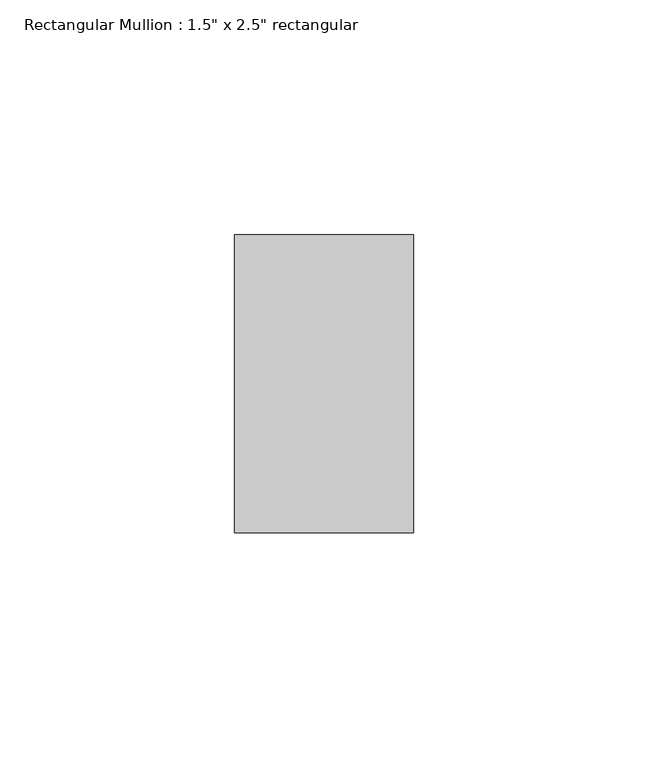
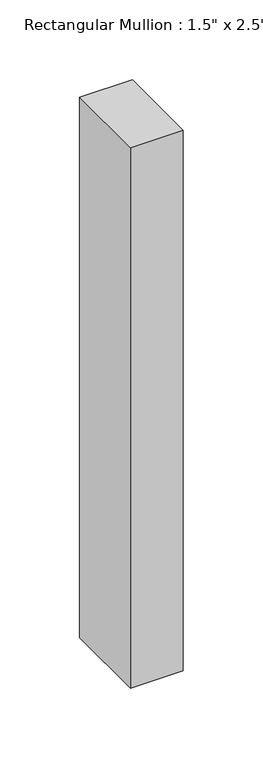
"""IFC4 building model written with IfcOpenShell, lengths in millimetres: member geometry."""

from ifc_helpers import new_model, si_unit, frame, origin, place, context, project, spatial, polyline, outline, extrude, source, transform, mapped, element, save


def member_f5dffbef(model_context):
    return source(origin(), model_context, "Body", "SweptSolid", [
        extrude(outline(polyline([(0.0, 31.75), (0.0, -31.75), (-38.1, -31.75), (-38.1, 31.75), (0.0, 31.75)])), frame((0.0, 0.0, -412.75), z_axis=(0.0, 0.0, 1.0), x_axis=(1.0, 0.0, 0.0)), (0.0, 0.0, 1.0), 412.75),
    ])


if __name__ == "__main__":
    model = new_model("IFC4")
    model_context = context("Model", 3, world=origin())
    ifc_project = project(units=[si_unit("LENGTHUNIT", "METRE", prefix="MILLI")], contexts=[model_context])
    site = spatial("IfcSite", under=ifc_project)
    building = spatial("IfcBuilding", under=site)
    placement = place(None, origin())
    member_shape = member_f5dffbef(model_context)
    element("IfcMember", 1, ObjectType="Rectangular Mullion : 1.5\" x 2.5\" rectangular", at=placement, inside=building, context=model_context, shape_type="MappedRepresentation", body=[
        mapped(member_shape, transform((0.0, 0.0, 0.0), x_axis=(1.0, 0.0, 0.0), y_axis=(0.0, 1.0, 0.0), z_axis=(0.0, 0.0, 1.0))),
    ])
    save(model, "model.ifc")

# Revit data of these elements
# Type "Rectangular Mullion : 1.5\" x 2.5\" rectangular"
#   built-in parameter 1007304 = 0.208333 (stored number, unit not read)
#   built-in parameter 1007301 = 0.0625 (stored number, unit not read)
#   built-in parameter 1007300 = 0.0625 (stored number, unit not read)
# Element 1 (IfcMember, "Rectangular Mullion : 1.5\" x 2.5\" rectangular")
#   Materials on its faces: "Aluminum"
# Materials
#   "Aluminum": class "Metal", colour RGB 247 247 247, transparency 0, Description = "Aluminum 6061", Cost = 0
